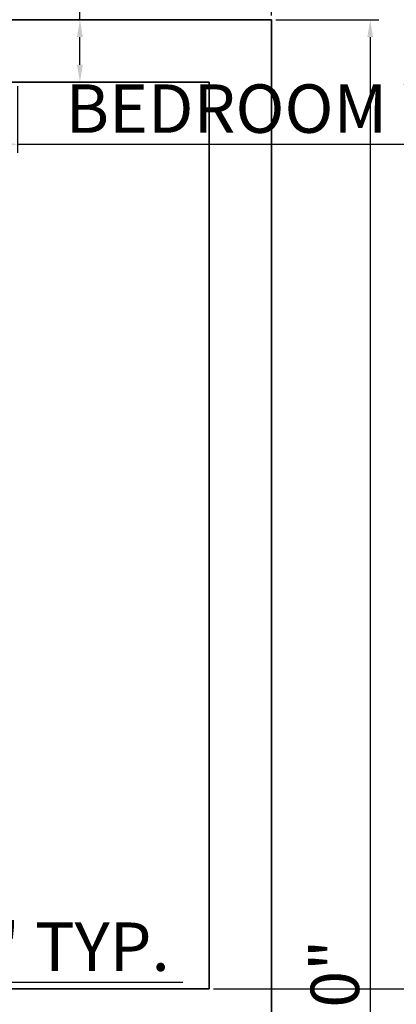
# Model space of a CAD drawing. Units: inches. Extents: x 1484 to 2008, y 1843 to 2590.
# Tile 18 of 21: x 1864 to 1918, y 2075 to 2217. Entities that reach past the tile are written whole.
import ezdxf

# ---------------------------------------------------------------- set-up
doc = ezdxf.new("R2010")
doc.units = ezdxf.units.IN
doc.layers.add('A-ANNO-DIMS', color=2, linetype='Continuous', lineweight=18)
doc.layers.add('A-WALL', color=7, linetype='Continuous', lineweight=35)
doc.styles.get("Standard").update_dxf_attribs({"font": 'arial.ttf'})
doc.dimstyles.new('ISO-25', dxfattribs={"dimtxt": 7, "dimasz": 2.5, "dimexe": 1.25, "dimexo": 0.625, "dimtad": 1, "dimdec": 0, "dimlunit": 3, "dimtxsty": 'Standard', "dimcen": 2.5, "dimadec": 0, "dimazin": 0, "dimtfac": 1, "dimtdec": 0, "dimtmove": 0, "dimatfit": 3, "dimfxl": 1, "dimarcsym": 0})

# ---------------------------------------------------------------- blocks, each defined once
blk = doc.blocks.new('*D2')
at = {"layer": 'A-ANNO-DIMS', "color": 0, "lineweight": -2, "transparency": 16777216}
for p, q in [((1602.92, 2217.93), (1602.92, 2236.39)), ((1899.92, 2217.93), (1899.92, 2236.39)), ((1605.42, 2235.14), (1897.42, 2235.14))]:
    blk.add_line(p, q, dxfattribs=at)
at = {"layer": 'A-ANNO-DIMS', "color": 0, "transparency": 16777216}
for points in [[(1605.42, 2235.55), (1605.42, 2234.72), (1602.92, 2235.14)], [(1897.42, 2235.55), (1897.42, 2234.72), (1899.92, 2235.14)]]:
    blk.add_solid(points, dxfattribs=at)
at = {"layer": 'Defpoints', "color": 0, "transparency": 16777216}
for p in [(1899.92, 2235.14), (1602.92, 2217.3), (1899.92, 2217.3)]:
    blk.add_point(p, dxfattribs=at)
at = {"layer": 'A-ANNO-DIMS', "color": 0, "transparency": 16777216, "insert": (1750.41, 2239.33), "char_height": 7, "attachment_point": 5}
blk.add_mtext('24\'-9"', dxfattribs=at)
blk = doc.blocks.new('*D3')
at = {"layer": 'A-ANNO-DIMS', "color": 0, "lineweight": -2, "transparency": 16777216}
for p, q in [((1900.54, 2217.3), (1915.42, 2217.3)), ((1914.17, 2214.8), (1914.17, 1922.3)), ((1900.54, 1919.8), (1915.42, 1919.8))]:
    blk.add_line(p, q, dxfattribs=at)
at = {"layer": 'A-ANNO-DIMS', "color": 0, "transparency": 16777216}
for points in [[(1913.75, 2214.8), (1914.58, 2214.8), (1914.17, 2217.3)], [(1913.75, 1922.3), (1914.58, 1922.3), (1914.17, 1919.8)]]:
    blk.add_solid(points, dxfattribs=at)
at = {"layer": 'Defpoints', "color": 0, "transparency": 16777216}
for p in [(1899.92, 2217.3), (1899.92, 1919.8), (1914.17, 1919.8)]:
    blk.add_point(p, dxfattribs=at)
at = {"layer": 'A-ANNO-DIMS', "color": 0, "transparency": 16777216, "insert": (1909.97, 2068.55), "char_height": 7, "attachment_point": 5, "rotation": 90}
blk.add_mtext('24\'-10"', dxfattribs=at)
blk = doc.blocks.new('*D11')
at = {"layer": 'A-ANNO-DIMS', "color": 0, "lineweight": -2, "transparency": 16777216}
for p, q in [((1754.42, 2083.34), (1754.42, 2076.98)), ((1792.67, 2083.34), (1792.67, 2076.98)), ((1756.92, 2078.23), (1790.17, 2078.23)), ((1792.67, 2078.23), (1887.1, 2078.23))]:
    blk.add_line(p, q, dxfattribs=at)
at = {"layer": 'A-ANNO-DIMS', "color": 0, "transparency": 16777216}
for points in [[(1756.92, 2078.64), (1756.92, 2077.81), (1754.42, 2078.23)], [(1790.17, 2078.64), (1790.17, 2077.81), (1792.67, 2078.23)]]:
    blk.add_solid(points, dxfattribs=at)
at = {"layer": 'Defpoints', "color": 0, "transparency": 16777216}
for p in [(1754.42, 2083.96), (1792.67, 2083.96), (1792.67, 2078.23)]:
    blk.add_point(p, dxfattribs=at)
at = {"layer": 'A-ANNO-DIMS', "color": 0, "transparency": 16777216, "insert": (1841.14, 2082.47), "char_height": 7, "attachment_point": 5}
blk.add_mtext('DOOR 3\'-2 1/2" TYP.', dxfattribs=at)
blk = doc.blocks.new('*D13')
at = {"layer": 'A-ANNO-DIMS', "color": 0, "lineweight": -2, "transparency": 16777216}
for p, q in [((1803.22, 2207.68), (1803.22, 2198.05)), ((1863.22, 2207.68), (1863.22, 2198.05)), ((1805.72, 2199.3), (1860.72, 2199.3)), ((1863.22, 2199.3), (2008.2, 2199.3))]:
    blk.add_line(p, q, dxfattribs=at)
at = {"layer": 'A-ANNO-DIMS', "color": 0, "transparency": 16777216}
for points in [[(1805.72, 2199.72), (1805.72, 2198.89), (1803.22, 2199.3)], [(1860.72, 2199.72), (1860.72, 2198.89), (1863.22, 2199.3)]]:
    blk.add_solid(points, dxfattribs=at)
at = {"layer": 'Defpoints', "color": 0, "transparency": 16777216}
for p in [(1803.22, 2208.3), (1863.22, 2208.3), (1863.22, 2199.3)]:
    blk.add_point(p, dxfattribs=at)
at = {"layer": 'A-ANNO-DIMS', "color": 0, "transparency": 16777216, "insert": (1936.96, 2203.55), "char_height": 7, "attachment_point": 5}
blk.add_mtext('BEDROOM WINDOW 5\'-0" TYP.', dxfattribs=at)
blk = doc.blocks.new('*D14')
at = {"layer": 'A-ANNO-DIMS', "color": 0, "lineweight": -2, "transparency": 16777216}
for p, q in [((1872.22, 2217.3), (1872.22, 2263.72)), ((1863.84, 2217.3), (1873.47, 2217.3)), ((1872.22, 2210.8), (1872.22, 2214.8)), ((1863.84, 2208.3), (1873.47, 2208.3))]:
    blk.add_line(p, q, dxfattribs=at)
at = {"layer": 'A-ANNO-DIMS', "color": 0, "transparency": 16777216}
for points in [[(1871.8, 2214.8), (1872.64, 2214.8), (1872.22, 2217.3)], [(1871.8, 2210.8), (1872.64, 2210.8), (1872.22, 2208.3)]]:
    blk.add_solid(points, dxfattribs=at)
at = {"layer": 'Defpoints', "color": 0, "transparency": 16777216}
for p in [(1863.22, 2217.3), (1872.22, 2217.3), (1863.22, 2208.3)]:
    blk.add_point(p, dxfattribs=at)
at = {"layer": 'A-ANNO-DIMS', "color": 0, "transparency": 16777216, "insert": (1868.02, 2241.76), "char_height": 7, "attachment_point": 5, "rotation": 90}
blk.add_mtext('0\'-9" TYP.', dxfattribs=at)
blk = doc.blocks.new('*D41')
at = {"layer": 'A-ANNO-DIMS', "color": 0, "lineweight": -2, "transparency": 16777216}
for p, q in [((1961.85, 2079.8), (1961.85, 2082.3)), ((1891.54, 2077.3), (1963.1, 2077.3)), ((1961.85, 2077.3), (1961.85, 2072.8)), ((1891.54, 2072.8), (1963.1, 2072.8)), ((1961.85, 2070.3), (1961.85, 2031.63))]:
    blk.add_line(p, q, dxfattribs=at)
at = {"layer": 'A-ANNO-DIMS', "color": 0, "transparency": 16777216}
for points in [[(1961.44, 2079.8), (1962.27, 2079.8), (1961.85, 2077.3)], [(1961.44, 2070.3), (1962.27, 2070.3), (1961.85, 2072.8)]]:
    blk.add_solid(points, dxfattribs=at)
at = {"layer": 'Defpoints', "color": 0, "transparency": 16777216}
for p in [(1890.92, 2077.3), (1890.92, 2072.8), (1961.85, 2072.8)]:
    blk.add_point(p, dxfattribs=at)
at = {"layer": 'A-ANNO-DIMS', "color": 0, "transparency": 16777216, "insert": (1957.61, 2049.72), "char_height": 7, "attachment_point": 5, "rotation": 90}
blk.add_mtext('0\'-4 1/2"', dxfattribs=at)

msp = doc.modelspace()

# ---------------------------------------------------------------- linework, layer by layer
at = {"layer": 'A-WALL'}
for p, q in [((1602.92, 2217.3), (1899.92, 2217.3)), ((1602.92, 2217.3), (1899.92, 2217.3)), ((1899.92, 2217.3), (1899.92, 1919.8)), ((1758.92, 2208.3), (1890.92, 2208.3)), ((1890.92, 2208.3), (1890.92, 2077.3)), ((1758.92, 2077.3), (1890.92, 2077.3))]:
    msp.add_line(p, q, dxfattribs=at)

# ---------------------------------------------------------------- dimensions: what is measured, and where the dimension line sits
at = {"layer": 'A-ANNO-DIMS'}
dim = msp.add_linear_dim(base=(1872.22, 2217.3), p1=(1863.22, 2208.3), p2=(1863.22, 2217.3), angle=90, text='<> TYP.', dimstyle='ISO-25', override={"dimdec": 1, "dimlfac": 1, "dimrnd": 0, "dimzin": 1, "dimdsep": 46, "dimlunit": 4, "dimfrac": 2}, dxfattribs=at)
dim.commit()
dim.dimension.update_dxf_attribs({"geometry": '*D14', "text_midpoint": (1868.02, 2241.76)})
dim = msp.add_linear_dim(base=(1899.92, 2235.14), p1=(1602.92, 2217.3), p2=(1899.92, 2217.3), dimstyle='ISO-25', override={"dimclrd": 0, "dimclre": 0, "dimclrt": 0}, dxfattribs=at)
dim.commit()
dim.dimension.update_dxf_attribs({"geometry": '*D2', "text_midpoint": (1750.41, 2235.14), "dimtype": 160})
for base, p1, p2, text, picture, middle in [((1863.22, 2199.3), (1803.22, 2208.3), (1863.22, 2208.3), 'BEDROOM WINDOW <> TYP.', '*D13', (1936.96, 2203.55)), ((1792.66964371, 2078.22557639), (1754.41964371, 2083.96307639), (1792.66964371, 2083.96307639), 'DOOR <> TYP.', '*D11', (1841.13707208, 2082.47472373))]:
    dim = msp.add_linear_dim(base=base, p1=p1, p2=p2, text=text, dimstyle='ISO-25', override={"dimdec": 1, "dimlfac": 1, "dimrnd": 0, "dimzin": 1, "dimdsep": 46, "dimlunit": 4, "dimfrac": 2}, dxfattribs=at)
    dim.commit()
    dim.dimension.update_dxf_attribs({"geometry": picture, "text_midpoint": middle})
for base, p1, p2, override, picture, middle in [((1914.166081, 1919.80284398), (1899.91964371, 2217.30284398), (1899.91964371, 1919.80284398), {"dimclrd": 0, "dimclre": 0, "dimclrt": 0}, '*D3', (1909.96707009, 2068.55284398)), ((1961.85, 2072.8), (1890.92, 2077.3), (1890.92, 2072.8), {"dimdec": 1, "dimlfac": 1, "dimrnd": 0, "dimzin": 1, "dimdsep": 46, "dimlunit": 4, "dimfrac": 2}, '*D41', (1957.61, 2049.72))]:
    dim = msp.add_linear_dim(base=base, p1=p1, p2=p2, angle=90, dimstyle='ISO-25', override=override, dxfattribs=at)
    dim.commit()
    dim.dimension.update_dxf_attribs({"geometry": picture, "text_midpoint": middle})

doc.saveas('drawing.dxf')
